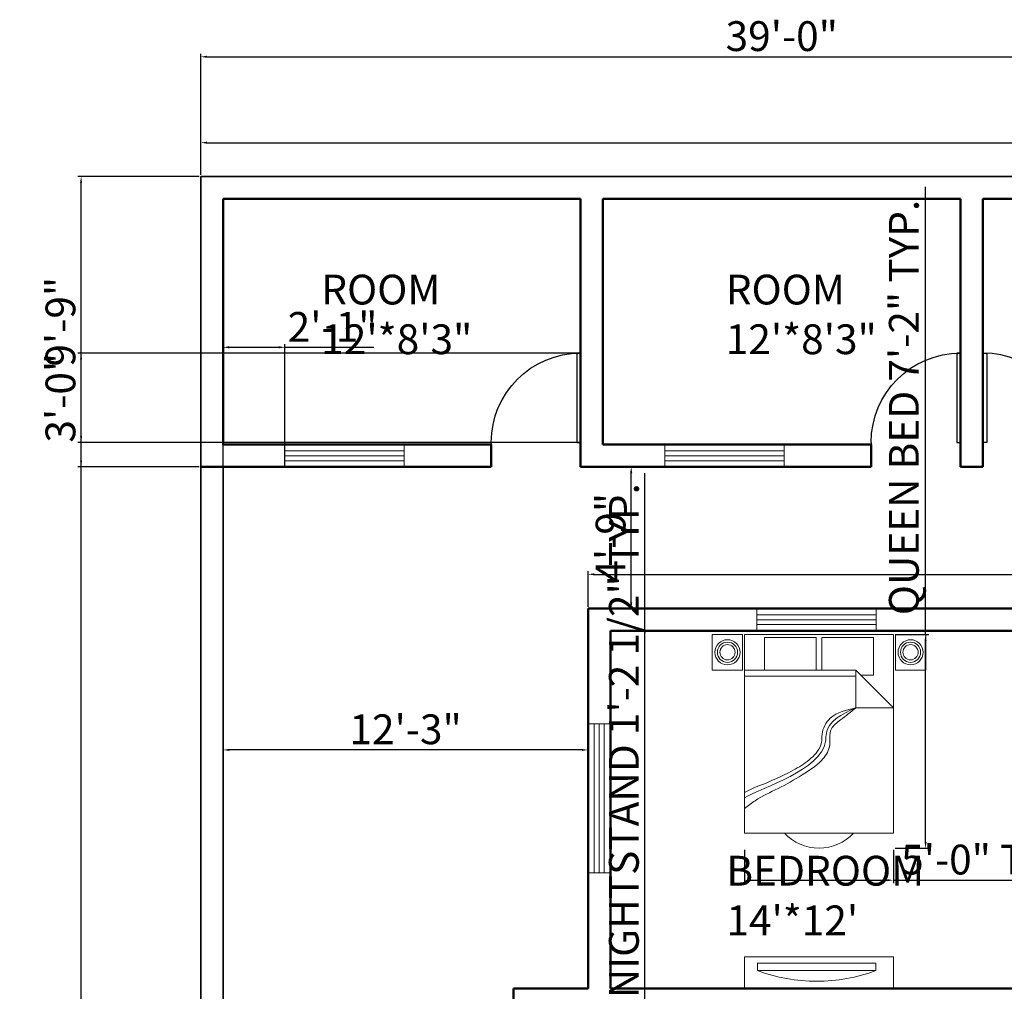
# Model space of a CAD drawing. Units: inches. Extents: x 6286 to 7213, y 5725 to 6776.
# Tile 4 of 5: x 6286 to 6683, y 6385 to 6776. Entities that reach past the tile are written whole.
import ezdxf

# ---------------------------------------------------------------- set-up
doc = ezdxf.new("R2010")
doc.units = ezdxf.units.IN
for name, color, linetype, lineweight in [('A-ANNO-DIMS', 2, 'Continuous', 18), ('A-AREA-IDEN', 7, 'Continuous', 25), ('A-DOOR', 3, 'Continuous', 25), ('A-FURN', 8, 'Continuous', 18), ('A-GLAZ', 4, 'Continuous', 18), ('A-WALL', 7, 'Continuous', 50), ('C-PROP', 7, 'Continuous', 35)]:
    doc.layers.add(name, color=color, linetype=linetype, lineweight=lineweight)
doc.styles.get("Standard").update_dxf_attribs({"font": 'arial.ttf'})
doc.dimstyles.new('ISO-25', dxfattribs={"dimtxt": 12, "dimasz": 2.5, "dimexe": 1.25, "dimexo": 0.625, "dimtad": 1, "dimdec": 1, "dimlunit": 4, "dimtxsty": 'Standard', "dimcen": 2.5, "dimadec": 0, "dimazin": 0, "dimtfac": 1, "dimtdec": 1, "dimtmove": 0, "dimatfit": 3, "dimfxl": 1, "dimarcsym": 0})

# ---------------------------------------------------------------- blocks, each defined once
blk = doc.blocks.new('*U2')
for p, q in [((0, 0), (0, -6)), ((40, 0), (40, -6))]:
    blk.add_line(p, q)
blk.add_lwpolyline([(0, 0), (0, 40), (1.75, 40), (1.75, 0)], close=True)
blk.add_arc((0, 0), 40, 0, 90)
blk = doc.blocks.new('*D3')
at = {"layer": 'A-ANNO-DIMS', "color": 0, "lineweight": -2, "transparency": 16777216}
for p, q in [((6358.92, 6713.89), (6358.92, 6728.11)), ((6361.42, 6726.86), (7061.42, 6726.86)), ((7063.92, 6713.89), (7063.92, 6728.11))]:
    blk.add_line(p, q, dxfattribs=at)
at = {"layer": 'A-ANNO-DIMS', "color": 0, "lineweight": 100, "transparency": 16777216}
for points in [[(6361.42, 6727.28), (6361.42, 6726.44), (6358.92, 6726.86)], [(7061.42, 6727.28), (7061.42, 6726.44), (7063.92, 6726.86)]]:
    blk.add_solid(points, dxfattribs=at)
at = {"layer": 'Defpoints', "color": 0, "lineweight": 100, "transparency": 16777216}
for p in [(7063.92, 6726.86), (6358.92, 6713.26), (7063.92, 6713.26)]:
    blk.add_point(p, dxfattribs=at)
at = {"layer": 'A-ANNO-DIMS', "color": 0, "transparency": 16777216, "insert": (6711.42, 6733.61), "char_height": 12, "attachment_point": 5}
blk.add_mtext('58\'-9"', dxfattribs=at)
blk = doc.blocks.new('*D4')
at = {"layer": 'A-ANNO-DIMS', "color": 0, "lineweight": -2, "transparency": 16777216}
for p, q in [((6515.55, 6596.26), (6533.53, 6596.26)), ((6532.28, 6541.76), (6532.28, 6593.76)), ((6515.55, 6539.26), (6533.53, 6539.26))]:
    blk.add_line(p, q, dxfattribs=at)
at = {"layer": 'A-ANNO-DIMS', "color": 0, "lineweight": 100, "transparency": 16777216}
for points in [[(6531.86, 6593.76), (6532.7, 6593.76), (6532.28, 6596.26)], [(6531.86, 6541.76), (6532.7, 6541.76), (6532.28, 6539.26)]]:
    blk.add_solid(points, dxfattribs=at)
at = {"layer": 'Defpoints', "color": 0, "lineweight": 100, "transparency": 16777216}
for p in [(6514.92, 6596.26), (6532.28, 6596.26), (6514.92, 6539.26)]:
    blk.add_point(p, dxfattribs=at)
at = {"layer": 'A-ANNO-DIMS', "color": 0, "transparency": 16777216, "insert": (6525.53, 6567.76), "char_height": 12, "attachment_point": 5, "rotation": 90}
blk.add_mtext('4\'-9"', dxfattribs=at)
blk = doc.blocks.new('*D5')
at = {"layer": 'A-ANNO-DIMS', "color": 0, "lineweight": -2, "transparency": 16777216}
for p, q in [((6514.92, 6539.89), (6514.92, 6554.27)), ((6517.42, 6553.02), (6980.42, 6553.02)), ((6982.92, 6539.89), (6982.92, 6554.27))]:
    blk.add_line(p, q, dxfattribs=at)
at = {"layer": 'A-ANNO-DIMS', "color": 0, "lineweight": 100, "transparency": 16777216}
for points in [[(6517.42, 6553.44), (6517.42, 6552.6), (6514.92, 6553.02)], [(6980.42, 6553.44), (6980.42, 6552.6), (6982.92, 6553.02)]]:
    blk.add_solid(points, dxfattribs=at)
at = {"layer": 'Defpoints', "color": 0, "lineweight": 100, "transparency": 16777216}
for p in [(6982.92, 6553.02), (6514.92, 6539.26), (6982.92, 6539.26)]:
    blk.add_point(p, dxfattribs=at)
at = {"layer": 'A-ANNO-DIMS', "color": 0, "transparency": 16777216, "insert": (6748.92, 6559.78), "char_height": 12, "attachment_point": 5}
blk.add_mtext("39'", dxfattribs=at)
blk = doc.blocks.new('*D6')
at = {"layer": 'A-ANNO-DIMS', "color": 0, "lineweight": -2, "transparency": 16777216}
for p, q in [((6367.92, 6538.64), (6367.92, 6481.05)), ((6514.92, 6538.64), (6514.92, 6481.05)), ((6512.42, 6482.3), (6370.42, 6482.3))]:
    blk.add_line(p, q, dxfattribs=at)
at = {"layer": 'A-ANNO-DIMS', "color": 0, "lineweight": 100, "transparency": 16777216}
for points in [[(6370.42, 6482.72), (6370.42, 6481.89), (6367.92, 6482.3)], [(6512.42, 6482.72), (6512.42, 6481.89), (6514.92, 6482.3)]]:
    blk.add_solid(points, dxfattribs=at)
at = {"layer": 'Defpoints', "color": 0, "lineweight": 100, "transparency": 16777216}
for p in [(6367.92, 6539.26), (6514.92, 6539.26), (6367.92, 6482.3)]:
    blk.add_point(p, dxfattribs=at)
at = {"layer": 'A-ANNO-DIMS', "color": 0, "transparency": 16777216, "insert": (6441.42, 6489.06), "char_height": 12, "attachment_point": 5}
blk.add_mtext('12\'-3"', dxfattribs=at)
blk = doc.blocks.new('*D25')
at = {"layer": 'A-ANNO-DIMS', "color": 0, "lineweight": -2, "transparency": 16777216}
for p, q in [((6367.92, 6385.64), (6367.92, 6360.28)), ((6484.92, 6385.64), (6484.92, 6360.28)), ((6482.42, 6361.53), (6370.42, 6361.53))]:
    blk.add_line(p, q, dxfattribs=at)
at = {"layer": 'A-ANNO-DIMS', "color": 0, "lineweight": 100, "transparency": 16777216}
for points in [[(6370.42, 6361.95), (6370.42, 6361.12), (6367.92, 6361.53)], [(6482.42, 6361.95), (6482.42, 6361.12), (6484.92, 6361.53)]]:
    blk.add_solid(points, dxfattribs=at)
at = {"layer": 'Defpoints', "color": 0, "lineweight": 100, "transparency": 16777216}
for p in [(6367.92, 6386.26), (6484.92, 6386.26), (6367.92, 6361.53)]:
    blk.add_point(p, dxfattribs=at)
at = {"layer": 'A-ANNO-DIMS', "color": 0, "transparency": 16777216, "insert": (6426.42, 6368.29), "char_height": 12, "attachment_point": 5}
blk.add_mtext('9\'-9"', dxfattribs=at)
blk = doc.blocks.new('WIN-48IN')
for p, q in [((0, 9), (0, 0)), ((48, 0), (48, 9)), ((0, 6.5), (48, 6.5)), ((0, 4.5), (48, 4.5)), ((0, 2.5), (48, 2.5))]:
    blk.add_line(p, q)
blk = doc.blocks.new('WIN-60IN')
for p, q in [((0, 9), (0, 0)), ((60, 0), (60, 9)), ((60, 6.5), (0, 6.5)), ((60, 4.5), (0, 4.5)), ((60, 2.5), (0, 2.5))]:
    blk.add_line(p, q)
blk = doc.blocks.new('NIGHTSTAND-LAMP')
blk.add_lwpolyline([(12.23, 14.4), (0, 14.4), (0, 0), (12.23, 0)], close=True)
for radius in [5.06, 4.06, 3.06]:
    blk.add_circle((6.12, 7.2), radius)
blk = doc.blocks.new('TV-CONSOLE-60IN')
for points in [[(0, 12.71), (60, 12.71), (60, 0), (0, 0)], [(5.19, 10.13), (52.94, 10.13), (52.94, 7.18), (5.19, 7.18)]]:
    blk.add_lwpolyline(points, close=True)
blk.add_arc((29.07, 71.71), 68.81, 249.6947, 290.3053)
blk = doc.blocks.new('Bed - Queen')
for p, q in [((0, -80.00003), (0, 0)), ((0, 0), (59.99999, 0)), ((59.99999, 0), (59.99999, -80.00003)), ((7.99999, -1.2), (28.79998, -1.2)), ((7.99999, -14.4), (7.99999, -1.2)), ((28.79998, -1.2), (28.79998, -14.4)), ((31.19999, -1.2), (51.99999, -1.2)), ((31.19999, -14.4), (31.19999, -1.2)), ((51.99999, -1.2), (51.99999, -16.4)), ((0, -14.4), (44.8, -14.4)), ((59.99999, -29.6), (44.8, -14.4)), ((44.8, -14.4), (44.8, -29.6)), ((44.8, -16.8), (0, -16.8)), ((51.99999, -16.4), (46.79936, -16.4)), ((44.8, -29.6), (59.99999, -29.6)), ((59.99999, -80.00003), (0, -80.00003))]:
    blk.add_line(p, q)
blk = doc.blocks.new('BED-QUEEN-DRESSED')
blk.add_arc((30, 18.96), 18.96, 222.7518, 317.2482)
for points, knots in [([(44.8, 56.49), (39.19, 53.96), (32.77, 51.07), (32.71, 32.08), (7.2, 24.53), (0, 20.27)], [0, 0, 0, 0, 16.08431, 18.417841, 48.068097, 48.068097, 48.068097, 48.068097]), ([(44.8, 56.49), (41.02, 55.65), (34.77, 54.26), (30.9, 47.2), (31.38, 41.03), (26.76, 35.63), (19.36, 31.03), (9.68, 26.38), (4.48, 24.69), (0, 22.46)], [0, 0, 0, 0, 11.066231, 18.341473, 21.645482, 29.256421, 37.126455, 49.94498, 57.001864, 57.001864, 57.001864, 57.001864]), ([(44.8, 56.49), (42.82, 54.88), (39.55, 52.2), (33.5, 47.94), (35.23, 40.79), (30.55, 34.13), (23.14, 29.37), (13.11, 23.54), (6.2, 20.75), (1.43, 17.09), (0, 16.03)], [0, 0, 0, 0, 7.83924, 12.978287, 20.287315, 26.568624, 36.127852, 46.548326, 57.45004, 62.118815, 62.118815, 62.118815, 62.118815])]:
    blk.add_open_spline(points, degree=3, knots=knots)
blk.add_blockref('Bed - Queen', (0, 86.09))
blk = doc.blocks.new('*D43')
at = {"layer": 'A-ANNO-DIMS', "color": 0, "lineweight": -2, "transparency": 16777216}
for p, q in [((6537.72, 6375.84), (6537.72, 6593.74)), ((6536.18, 6375.84), (6538.97, 6375.84)), ((6537.72, 6363.94), (6537.72, 6373.34)), ((6536.18, 6361.44), (6538.97, 6361.44))]:
    blk.add_line(p, q, dxfattribs=at)
at = {"layer": 'A-ANNO-DIMS', "color": 0, "lineweight": 100, "transparency": 16777216}
for points in [[(6537.3, 6373.34), (6538.13, 6373.34), (6537.72, 6375.84)], [(6537.3, 6363.94), (6538.13, 6363.94), (6537.72, 6361.44)]]:
    blk.add_solid(points, dxfattribs=at)
at = {"layer": 'Defpoints', "color": 0, "lineweight": 100, "transparency": 16777216}
for p in [(6535.56, 6375.84), (6537.72, 6375.84), (6535.56, 6361.44)]:
    blk.add_point(p, dxfattribs=at)
at = {"layer": 'A-ANNO-DIMS', "color": 0, "transparency": 16777216, "insert": (6530.89, 6486.04), "char_height": 12, "attachment_point": 5, "rotation": 90}
blk.add_mtext('NIGHTSTAND 1\'-2 1/2" TYP.', dxfattribs=at)
blk = doc.blocks.new('*D47')
at = {"layer": 'A-ANNO-DIMS', "color": 0, "lineweight": -2, "transparency": 16777216}
for p, q in [((6650.84, 6528.84), (6650.84, 6709.11)), ((6638.55, 6528.84), (6652.09, 6528.84)), ((6650.84, 6445.25), (6650.84, 6526.34)), ((6638.55, 6442.75), (6652.09, 6442.75))]:
    blk.add_line(p, q, dxfattribs=at)
at = {"layer": 'A-ANNO-DIMS', "color": 0, "lineweight": 100, "transparency": 16777216}
for points in [[(6650.42, 6526.34), (6651.25, 6526.34), (6650.84, 6528.84)], [(6650.42, 6445.25), (6651.25, 6445.25), (6650.84, 6442.75)]]:
    blk.add_solid(points, dxfattribs=at)
at = {"layer": 'Defpoints', "color": 0, "lineweight": 100, "transparency": 16777216}
for p in [(6637.92, 6528.84), (6650.84, 6528.84), (6637.92, 6442.75)]:
    blk.add_point(p, dxfattribs=at)
at = {"layer": 'A-ANNO-DIMS', "color": 0, "transparency": 16777216, "insert": (6643.64, 6620.22), "char_height": 12, "attachment_point": 5, "rotation": 90}
blk.add_mtext('QUEEN BED 7\'-2" TYP.', dxfattribs=at)
blk = doc.blocks.new('*D48')
at = {"layer": 'A-ANNO-DIMS', "color": 0, "lineweight": -2, "transparency": 16777216}
for p, q in [((6577.92, 6442.12), (6577.92, 6428.58)), ((6637.92, 6442.12), (6637.92, 6428.58)), ((6580.42, 6429.83), (6635.42, 6429.83)), ((6637.92, 6429.83), (6714.82, 6429.83))]:
    blk.add_line(p, q, dxfattribs=at)
at = {"layer": 'A-ANNO-DIMS', "color": 0, "lineweight": 100, "transparency": 16777216}
for points in [[(6580.42, 6430.25), (6580.42, 6429.42), (6577.92, 6429.83)], [(6635.42, 6430.25), (6635.42, 6429.42), (6637.92, 6429.83)]]:
    blk.add_solid(points, dxfattribs=at)
at = {"layer": 'Defpoints', "color": 0, "lineweight": 100, "transparency": 16777216}
for p in [(6577.92, 6442.75), (6637.92, 6442.75), (6637.92, 6429.83)]:
    blk.add_point(p, dxfattribs=at)
at = {"layer": 'A-ANNO-DIMS', "color": 0, "transparency": 16777216, "insert": (6677.62, 6436.59), "char_height": 12, "attachment_point": 5}
blk.add_mtext('5\'-0" TYP.', dxfattribs=at)
blk = doc.blocks.new('*D55')
at = {"layer": 'A-ANNO-DIMS', "color": 0, "lineweight": -2, "transparency": 16777216}
for p, q in [((6358.3, 6713.26), (6309.47, 6713.26)), ((6310.72, 6598.76), (6310.72, 6710.76)), ((6358.3, 6596.26), (6309.47, 6596.26))]:
    blk.add_line(p, q, dxfattribs=at)
at = {"layer": 'A-ANNO-DIMS', "color": 0, "lineweight": 100, "transparency": 16777216}
for points in [[(6310.31, 6710.76), (6311.14, 6710.76), (6310.72, 6713.26)], [(6310.31, 6598.76), (6311.14, 6598.76), (6310.72, 6596.26)]]:
    blk.add_solid(points, dxfattribs=at)
at = {"layer": 'Defpoints', "color": 0, "lineweight": 100, "transparency": 16777216}
for p in [(6310.72, 6713.26), (6358.92, 6713.26), (6358.92, 6596.26)]:
    blk.add_point(p, dxfattribs=at)
at = {"layer": 'A-ANNO-DIMS', "color": 0, "transparency": 16777216, "insert": (6303.97, 6654.76), "char_height": 12, "attachment_point": 5, "rotation": 90}
blk.add_mtext('9\'-9"', dxfattribs=at)
blk = doc.blocks.new('*D56')
at = {"layer": 'A-ANNO-DIMS', "color": 0, "lineweight": -2, "transparency": 16777216}
for p, q in [((6358.3, 6713.26), (6309.47, 6713.26)), ((6310.72, 5787.26), (6310.72, 6710.76)), ((6358.3, 5784.76), (6309.47, 5784.76))]:
    blk.add_line(p, q, dxfattribs=at)
at = {"layer": 'A-ANNO-DIMS', "color": 0, "lineweight": 100, "transparency": 16777216}
for points in [[(6310.31, 6710.76), (6311.14, 6710.76), (6310.72, 6713.26)], [(6310.31, 5787.26), (6311.14, 5787.26), (6310.72, 5784.76)]]:
    blk.add_solid(points, dxfattribs=at)
at = {"layer": 'Defpoints', "color": 0, "lineweight": 100, "transparency": 16777216}
for p in [(6310.72, 6713.26), (6358.92, 6713.26), (6358.92, 5784.76)]:
    blk.add_point(p, dxfattribs=at)
at = {"layer": 'A-ANNO-DIMS', "color": 0, "transparency": 16777216, "insert": (6303.89, 6249.01), "char_height": 12, "attachment_point": 5, "rotation": 90}
blk.add_mtext('77\'-4 1/2"', dxfattribs=at)
blk = doc.blocks.new('*D57')
at = {"layer": 'A-ANNO-DIMS', "color": 0, "lineweight": -2, "transparency": 16777216}
for p, q in [((6358.92, 6713.89), (6358.92, 6762.71)), ((6361.42, 6761.46), (6824.42, 6761.46)), ((6826.92, 6704.89), (6826.92, 6762.71))]:
    blk.add_line(p, q, dxfattribs=at)
at = {"layer": 'A-ANNO-DIMS', "color": 0, "lineweight": 100, "transparency": 16777216}
for points in [[(6361.42, 6761.88), (6361.42, 6761.05), (6358.92, 6761.46)], [(6824.42, 6761.88), (6824.42, 6761.05), (6826.92, 6761.46)]]:
    blk.add_solid(points, dxfattribs=at)
at = {"layer": 'Defpoints', "color": 0, "lineweight": 100, "transparency": 16777216}
for p in [(6826.92, 6761.46), (6358.92, 6713.26), (6826.92, 6704.26)]:
    blk.add_point(p, dxfattribs=at)
at = {"layer": 'A-ANNO-DIMS', "color": 0, "transparency": 16777216, "insert": (6592.92, 6768.22), "char_height": 12, "attachment_point": 5}
blk.add_mtext('39\'-0"', dxfattribs=at)
blk = doc.blocks.new('*D67')
at = {"layer": 'A-ANNO-DIMS', "color": 0, "lineweight": -2, "transparency": 16777216}
for p, q in [((6511.3, 6642.16), (6309.47, 6642.16)), ((6310.72, 6608.66), (6310.72, 6639.66)), ((6511.3, 6606.16), (6309.47, 6606.16))]:
    blk.add_line(p, q, dxfattribs=at)
at = {"layer": 'A-ANNO-DIMS', "color": 0, "lineweight": 100, "transparency": 16777216}
for points in [[(6310.31, 6639.66), (6311.14, 6639.66), (6310.72, 6642.16)], [(6310.31, 6608.66), (6311.14, 6608.66), (6310.72, 6606.16)]]:
    blk.add_solid(points, dxfattribs=at)
at = {"layer": 'Defpoints', "color": 0, "lineweight": 100, "transparency": 16777216}
for p in [(6310.72, 6642.16), (6511.92, 6642.16), (6511.92, 6606.16)]:
    blk.add_point(p, dxfattribs=at)
at = {"layer": 'A-ANNO-DIMS', "color": 0, "transparency": 16777216, "insert": (6303.97, 6624.16), "char_height": 12, "attachment_point": 5, "rotation": 90}
blk.add_mtext('3\'-0"', dxfattribs=at)
blk = doc.blocks.new('*D73')
at = {"layer": 'A-ANNO-DIMS', "color": 0, "lineweight": -2, "transparency": 16777216}
for p, q in [((6367.92, 6596.89), (6367.92, 6645.71)), ((6370.42, 6644.46), (6390.33, 6644.46)), ((6392.83, 6596.89), (6392.83, 6645.71)), ((6392.83, 6644.46), (6428.68, 6644.46))]:
    blk.add_line(p, q, dxfattribs=at)
at = {"layer": 'A-ANNO-DIMS', "color": 0, "lineweight": 100, "transparency": 16777216}
for points in [[(6370.42, 6644.88), (6370.42, 6644.05), (6367.92, 6644.46)], [(6390.33, 6644.88), (6390.33, 6644.05), (6392.83, 6644.46)]]:
    blk.add_solid(points, dxfattribs=at)
at = {"layer": 'Defpoints', "color": 0, "lineweight": 100, "transparency": 16777216}
for p in [(6392.83, 6644.46), (6367.92, 6596.26), (6392.83, 6596.26)]:
    blk.add_point(p, dxfattribs=at)
at = {"layer": 'A-ANNO-DIMS', "color": 0, "transparency": 16777216, "insert": (6412, 6651.11), "char_height": 12, "attachment_point": 5}
blk.add_mtext('2\'-1"', dxfattribs=at)

msp = doc.modelspace()

# ---------------------------------------------------------------- linework, layer by layer
at = {"layer": 'A-WALL'}
for p, q in [((6367.92, 6704.26), (6367.92, 6605.26)), ((6367.92, 6704.26), (6511.92, 6704.26)), ((6511.92, 6704.26), (6511.92, 6596.26)), ((6520.92, 6704.26), (6520.92, 6605.26)), ((6520.92, 6704.26), (6664.92, 6704.26)), ((6664.92, 6704.26), (6664.92, 6596.26)), ((6673.92, 6704.26), (6673.92, 6596.26)), ((6673.92, 6704.26), (6817.92, 6704.26)), ((6367.92, 6605.26), (6475.92, 6605.26)), ((6475.92, 6605.26), (6475.92, 6596.26)), ((6520.92, 6605.26), (6628.94, 6605.26)), ((6628.94, 6605.26), (6628.94, 6596.26)), ((6358.92, 6596.26), (6475.92, 6596.26)), ((6511.92, 6596.26), (6628.94, 6596.26)), ((6664.92, 6596.26), (6673.92, 6596.26)), ((6514.92, 6539.26), (6514.92, 6386.26)), ((6514.92, 6539.26), (6982.92, 6539.26)), ((6523.92, 6530.26), (6523.92, 6386.26)), ((6523.92, 6530.26), (6691.92, 6530.26)), ((6514.92, 6386.26), (6484.92, 6386.26)), ((6484.92, 6386.26), (6484.92, 6377.26)), ((6838.92, 6386.26), (6523.92, 6386.26))]:
    msp.add_line(p, q, dxfattribs=at)
at = {"layer": 'C-PROP'}
for p, q in [((6358.92, 6713.26), (7063.92, 6713.26)), ((6358.92, 6713.26), (6358.92, 5784.76)), ((6367.92, 6596.26), (6367.92, 5793.76))]:
    msp.add_line(p, q, dxfattribs=at)

# ---------------------------------------------------------------- block references
at = {"layer": 'A-DOOR', "yscale": 0.9, "zscale": 0.9}
for p, xscale in [((6511.92, 6606.16), -0.9), ((6664.94, 6606.16), -0.9), ((6673.92, 6606.16), 0.9)]:
    msp.add_blockref('*U2', p, dxfattribs=dict(at, xscale=xscale))
at = {"layer": 'A-FURN'}
for name, p in [('NIGHTSTAND-LAMP', (6564.93, 6514.44)), ('BED-QUEEN-DRESSED', (6577.92, 6442.75)), ('TV-CONSOLE-60IN', (6577.92, 6386.26))]:
    msp.add_blockref(name, p, dxfattribs=at)
at = {"layer": 'A-FURN', "extrusion": (0, 0, -1), "zscale": -1}
msp.add_blockref('NIGHTSTAND-LAMP', (-6650.92, 6514.44), dxfattribs=at)
at = {"layer": 'A-GLAZ'}
for p in [(6392.83, 6596.26), (6545.83, 6596.26), (6582.94, 6530.26)]:
    msp.add_blockref('WIN-48IN', p, dxfattribs=at)
at = {"layer": 'A-GLAZ', "rotation": 89.99999999999714}
msp.add_blockref('WIN-60IN', (6523.92, 6432.76), dxfattribs=at)

# ---------------------------------------------------------------- texts
at = {"layer": 'A-AREA-IDEN', "char_height": 12, "attachment_point": 1}
for s, width, insert in [('ROOM\\P12\'*8\'3"', 50.4215, (6407.45, 6673.7)), ('ROOM\\P12\'*8\'3"', 50.4215, (6570.36, 6673.7)), ("BEDROOM\\P14'*12'", 61.4508, (6570.62, 6439.66))]:
    msp.add_mtext_dynamic_manual_height_columns(s, width=width, gutter_width=12.5, heights=[0], dxfattribs=dict(at, insert=insert))

# ---------------------------------------------------------------- dimensions: what is measured, and where the dimension line sits
at = {"layer": 'A-ANNO-DIMS'}
for base, p1, p2, override, picture, middle in [((6826.92, 6761.46), (6358.92, 6713.26), (6826.92, 6704.26), {"dimdec": 1, "dimlfac": 1, "dimrnd": 0, "dimzin": 1, "dimdsep": 46, "dimlunit": 4, "dimfrac": 2}, '*D57', (6592.92, 6768.22)), ((7063.92, 6726.86), (6358.92, 6713.26), (7063.92, 6713.26), {"dimclrd": 0, "dimclre": 0, "dimclrt": 0}, '*D3', (6711.42, 6733.61)), ((6982.92, 6553.02), (6514.92, 6539.26), (6982.92, 6539.26), {"dimclrd": 0, "dimclre": 0, "dimclrt": 0}, '*D5', (6748.92, 6559.78)), ((6367.92, 6482.3), (6514.92, 6539.26), (6367.92, 6539.26), {"dimclrd": 0, "dimclre": 0, "dimclrt": 0}, '*D6', (6441.42, 6489.06)), ((6367.92, 6361.53), (6484.92, 6386.26), (6367.92, 6386.26), {"dimclrd": 0, "dimclre": 0, "dimclrt": 0}, '*D25', (6426.42, 6368.29))]:
    dim = msp.add_linear_dim(base=base, p1=p1, p2=p2, dimstyle='ISO-25', override=override, dxfattribs=at)
    dim.commit()
    dim.dimension.update_dxf_attribs({"geometry": picture, "text_midpoint": middle})
for base, p1, p2, angle, override, picture, middle in [((6310.72, 6713.26), (6358.92, 5784.76), (6358.92, 6713.26), 90, {"dimdec": 1, "dimlfac": 1, "dimrnd": 0, "dimzin": 1, "dimdsep": 46, "dimlunit": 4, "dimfrac": 2}, '*D56', (6303.89, 6249.01)), ((6310.72, 6713.26), (6358.92, 6596.26), (6358.92, 6713.26), 90, {"dimdec": 1, "dimlfac": 1, "dimrnd": 0, "dimzin": 1, "dimdsep": 46, "dimlunit": 4, "dimfrac": 2}, '*D55', (6303.97, 6654.76)), ((6392.83, 6644.46), (6367.92, 6596.26), (6392.83, 6596.26), 0, {"dimdec": 1, "dimlfac": 1, "dimrnd": 0, "dimzin": 1, "dimdsep": 46, "dimlunit": 4, "dimfrac": 2}, '*D73', (6412, 6651.11)), ((6310.72, 6642.16), (6511.92, 6606.16), (6511.92, 6642.16), 90, {"dimdec": 1, "dimlfac": 1, "dimrnd": 0, "dimzin": 1, "dimdsep": 46, "dimlunit": 4, "dimfrac": 2}, '*D67', (6303.97, 6624.16)), ((6532.28, 6596.26), (6514.92, 6539.26), (6514.92, 6596.26), 90, {"dimclrd": 0, "dimclre": 0, "dimclrt": 0}, '*D4', (6525.53, 6567.76))]:
    dim = msp.add_linear_dim(base=base, p1=p1, p2=p2, angle=angle, dimstyle='ISO-25', override=override, dxfattribs=at)
    dim.commit()
    dim.dimension.update_dxf_attribs({"geometry": picture, "text_midpoint": middle})
for base, p1, p2, text, picture, middle in [((6650.84, 6528.84), (6637.92, 6442.75), (6637.92, 6528.84), 'QUEEN BED <> TYP.', '*D47', (6643.64, 6620.22)), ((6537.72, 6375.84), (6535.56, 6361.44), (6535.56, 6375.84), 'NIGHTSTAND <> TYP.', '*D43', (6530.89, 6486.04))]:
    dim = msp.add_linear_dim(base=base, p1=p1, p2=p2, angle=90, text=text, dimstyle='ISO-25', override={"dimdec": 1, "dimlfac": 1, "dimrnd": 0, "dimzin": 1, "dimdsep": 46, "dimlunit": 4, "dimfrac": 2}, dxfattribs=at)
    dim.commit()
    dim.dimension.update_dxf_attribs({"geometry": picture, "text_midpoint": middle})
dim = msp.add_linear_dim(base=(6637.92, 6429.83), p1=(6577.92, 6442.75), p2=(6637.92, 6442.75), text='<> TYP.', dimstyle='ISO-25', override={"dimdec": 1, "dimlfac": 1, "dimrnd": 0, "dimzin": 1, "dimdsep": 46, "dimlunit": 4, "dimfrac": 2}, dxfattribs=at)
dim.commit()
dim.dimension.update_dxf_attribs({"geometry": '*D48', "text_midpoint": (6677.62, 6436.59)})

doc.saveas('drawing.dxf')
